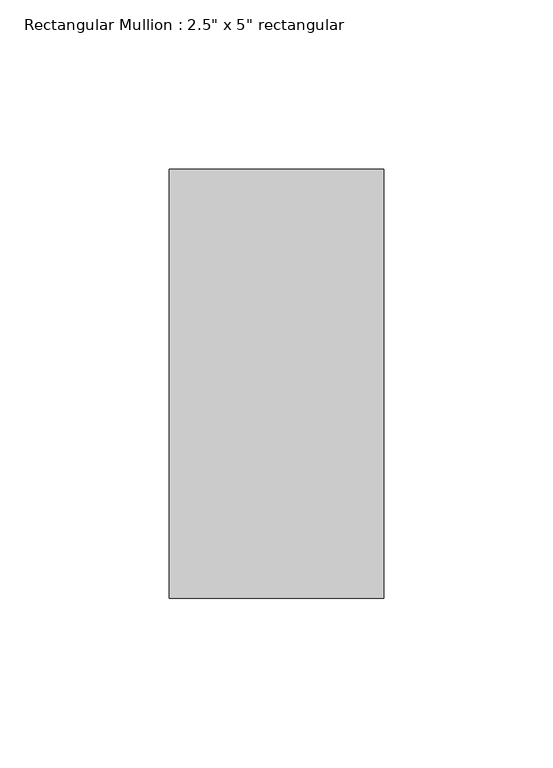
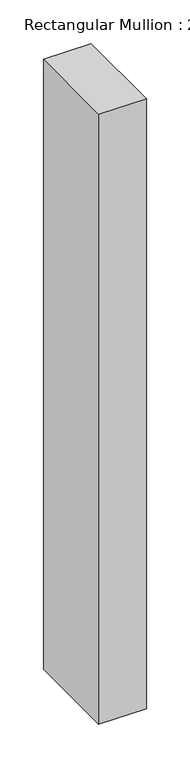
"""IFC4 building model written with IfcOpenShell, lengths in millimetres: member geometry."""

from ifc_helpers import new_model, si_unit, frame, origin, place, context, project, spatial, polyline, outline, extrude, source, transform, mapped, element, save


def member_c60babaf(model_context):
    return source(origin(), model_context, "Body", "SweptSolid", [
        extrude(outline(polyline([(0.0, 63.5), (0.0, -63.5), (-63.5, -63.5), (-63.5, 63.5), (0.0, 63.5)])), frame((0.0, 0.0, -854.843224), z_axis=(0.0, 0.0, 1.0), x_axis=(1.0, 0.0, 0.0)), (0.0, 0.0, 1.0), 854.843224),
    ])


if __name__ == "__main__":
    model = new_model("IFC4")
    model_context = context("Model", 3, world=origin())
    ifc_project = project(units=[si_unit("LENGTHUNIT", "METRE", prefix="MILLI")], contexts=[model_context])
    site = spatial("IfcSite", under=ifc_project)
    building = spatial("IfcBuilding", under=site)
    placement = place(None, origin())
    member_shape = member_c60babaf(model_context)
    element("IfcMember", 1, ObjectType="Rectangular Mullion : 2.5\" x 5\" rectangular", at=placement, inside=building, context=model_context, shape_type="MappedRepresentation", body=[
        mapped(member_shape, transform((0.0, 0.0, 0.0), x_axis=(1.0, 0.0, 0.0), y_axis=(0.0, 1.0, 0.0), z_axis=(0.0, 0.0, 1.0))),
    ])
    save(model, "model.ifc")

# Revit data of these elements
# Type "Rectangular Mullion : 2.5\" x 5\" rectangular"
#   built-in parameter 1007304 = 0.416667 (stored number, unit not read)
#   built-in parameter 1007301 = 0.104167 (stored number, unit not read)
#   built-in parameter 1007300 = 0.104167 (stored number, unit not read)
# Element 1 (IfcMember, "Rectangular Mullion : 2.5\" x 5\" rectangular")
#   Materials on its faces: "Aluminum"
# Materials
#   "Aluminum": class "Metal", colour RGB 247 247 247, transparency 0, Description = "Aluminum 6061", Cost = 0
